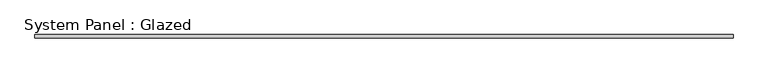
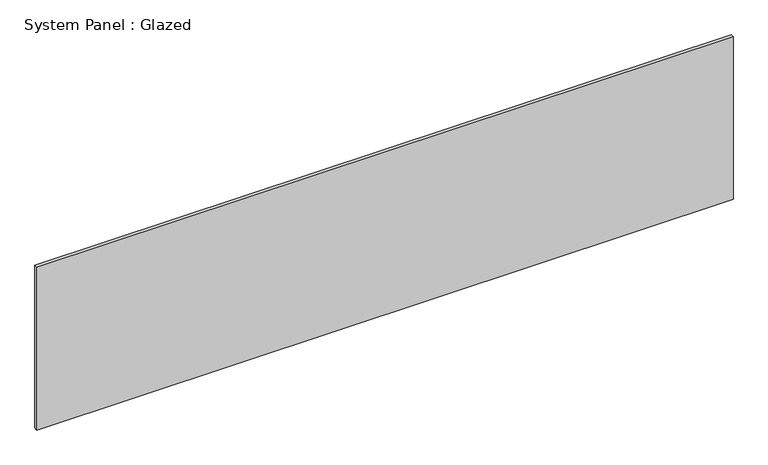
"""IFC4 building model written with IfcOpenShell, lengths in millimetres: plate geometry, System Panel : Glazed."""

from ifc_helpers import new_model, si_unit, origin, origin_with_axes, place, context, project, spatial, polyline, outline, extrude, source, transform, mapped, element, save


def system_panel_glazed_773201f3(model_context):
    return source(origin(), model_context, "Body", "SweptSolid", [
        extrude(outline(polyline([(2469.7006486, 19.05), (-2469.7006486, 19.05), (-2469.7006486, 44.45), (2469.7006486, 44.45), (2469.7006486, 19.05)])), origin_with_axes(), (0.0, 0.0, 1.0), 1219.2),
    ])


if __name__ == "__main__":
    model = new_model("IFC4")
    model_context = context("Model", 3, world=origin())
    ifc_project = project(units=[si_unit("LENGTHUNIT", "METRE", prefix="MILLI")], contexts=[model_context])
    site = spatial("IfcSite", under=ifc_project)
    building = spatial("IfcBuilding", under=site)
    placement = place(None, origin())
    system_panel_glazed_shape = system_panel_glazed_773201f3(model_context)
    element("IfcPlate", 1, ObjectType="System Panel : Glazed", at=placement, inside=building, context=model_context, shape_type="MappedRepresentation", body=[
        mapped(system_panel_glazed_shape, transform((0.0, 0.0, 0.0), x_axis=(1.0, 0.0, 0.0), y_axis=(0.0, 1.0, 0.0), z_axis=(0.0, 0.0, 1.0))),
    ])
    save(model, "model.ifc")

# Revit data of these elements
# Type "System Panel : Glazed"
#   Construction Type Id = "GSP4R"
#   Analytic Construction = "1/8 in Pilkington single glazing"
#   Visual Light Transmittance = 0.9
#   Solar Heat Gain Coefficient = 0.86
#   Heat Transfer Coefficient (U) = 1.18115 BTU/(h·ft²·°F)
# Element 1 (IfcPlate, "System Panel : Glazed")
#   Materials on its faces: "Glass"
# Materials
#   "Glass": class "Glass", colour RGB 0 128 192, transparency 0.75, Description = "Soda Lime Glass", Cost = 0
